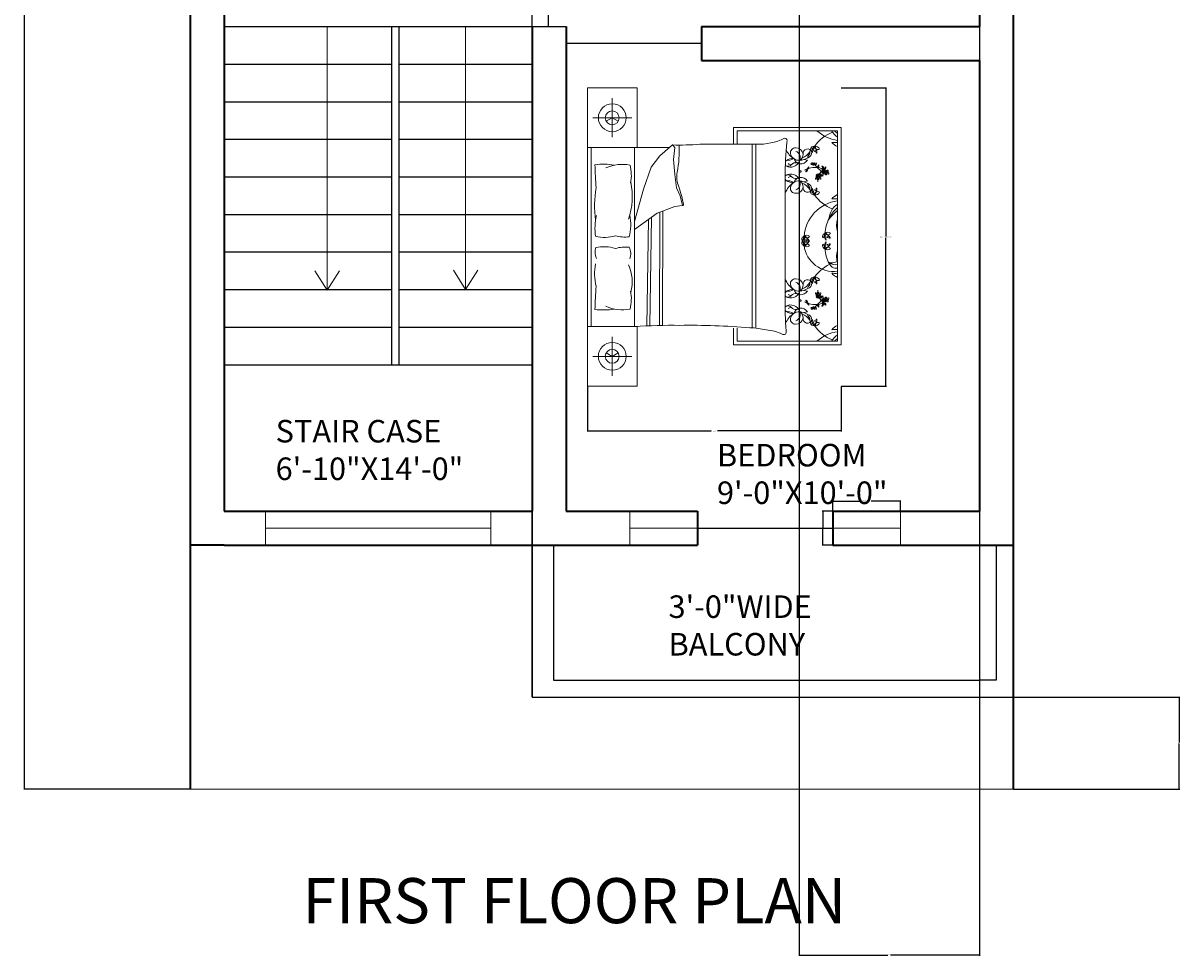
# Model space of a CAD drawing. Units: inches. Extents: x -16 to 587, y -783 to 64.
# Tile 8 of 14: x 279 to 587, y -782 to -534. Entities that reach past the tile are written whole.
import ezdxf

# ---------------------------------------------------------------- set-up
doc = ezdxf.new("R2010")
doc.units = ezdxf.units.IN
doc.header["$MEASUREMENT"] = 0
for name, color, linetype, lineweight in [('A-ANNO-DIMS', 2, 'Continuous', 18), ('A-ANNO-SYMB', 7, 'Continuous', 18), ('A-ANNO-TEXT', 7, 'Continuous', 25), ('A-AREA-IDEN', 7, 'Continuous', 18), ('A-DOOR', 3, 'Continuous', 25), ('A-FLOR-BALC', 7, 'Continuous', 25), ('A-FLOR-STRS', 7, 'Continuous', 25), ('A-FURN', 8, 'Continuous', 18), ('A-GLAZ', 4, 'Continuous', 18), ('A-WALL', 7, 'Continuous', 35), ('C-PROP', 7, 'Continuous', 18)]:
    doc.layers.add(name, color=color, linetype=linetype, lineweight=lineweight)
doc.styles.get("Standard").update_dxf_attribs({"font": 'arial.ttf'})
doc.dimstyles.get("Standard").update_dxf_attribs({"dimtxt": 0.18, "dimasz": 0.18, "dimexe": 0.18, "dimexo": 0.0625, "dimgap": 0.09, "dimtad": 0, "dimtih": 1, "dimtoh": 1, "dimdec": 0, "dimzin": 0, "dimdsep": 46, "dimlunit": 3, "dimtxsty": 'Standard', "dimcen": 0.09, "dimadec": 0, "dimazin": 0, "dimtfac": 1, "dimtdec": 0, "dimtofl": 0, "dimtmove": 0, "dimatfit": 3, "dimfxl": 1, "dimtolj": 1, "dimtzin": 0, "dimarcsym": 0})

# ---------------------------------------------------------------- blocks, each defined once
blk = doc.blocks.new('BED-DOUBLE-COMPACT')
for p, q in [((0, 79.37), (0, 0)), ((6.61, 66.25), (6.61, 76.62)), ((11.8, 71.43), (1.43, 71.43)), ((38.91, 68.89), (38.91, 64.4)), ((67.5, 68.89), (38.91, 68.89)), ((39.83, 64.41), (39.83, 67.97)), ((39.83, 67.97), (66.58, 67.97)), ((66.58, 67.97), (66.58, 11.95)), ((67.5, 11.03), (67.5, 68.89)), ((0, 63.5), (21.78, 63.5)), ((1.02, 15.87), (1.02, 63.5)), ((12.54, 63.5), (12.54, 15.87)), ((22.61, 64.21), (19.24, 61.31)), ((23.26, 63.56), (22.61, 64.21)), ((22.93, 60.35), (23.26, 63.56)), ((43.86, 15.51), (43.86, 64.41)), ((44.85, 15.44), (44.85, 64.41)), ((19.24, 61.31), (16.99, 58.26)), ((23.26, 56.33), (22.93, 60.35)), ((58.53, 60.15), (57.63, 60.33)), ((16.99, 58.26), (14.9, 52.47)), ((23.74, 52.79), (23.26, 56.33)), ((52.64, 23.57), (52.64, 55.8)), ((14.9, 52.47), (12.54, 43.82)), ((24.7, 50.7), (23.74, 52.79)), ((58.53, 54.61), (57.63, 54.43)), ((25.34, 48.13), (24.7, 50.7)), ((18.6, 46.04), (23.26, 47.81)), ((19.15, 16.16), (19.27, 46.3)), ((19.97, 16.15), (20.09, 46.61)), ((23.26, 47.81), (25.34, 48.13)), ((12.54, 41.69), (18.6, 46.04)), ((15.84, 16.09), (16.24, 44.34)), ((16.65, 16.12), (17.06, 44.94)), ((58.53, 25.32), (57.63, 25.49)), ((58.53, 19.77), (57.63, 19.6)), ((38.91, 15.43), (38.91, 11.03)), ((39.83, 11.95), (39.83, 15.45)), ((6.61, 13.12), (6.61, 2.75)), ((38.91, 11.03), (67.5, 11.03)), ((66.58, 11.95), (39.83, 11.95)), ((11.8, 7.94), (1.43, 7.94))]:
    blk.add_line(p, q)
for points in [[(13.23, 63.5), (13.23, 79.37), (0, 79.37)], [(6.61, 71.43), (5.01, 70.51)], [(6.61, 71.43), (8.22, 70.51)], [(0, 15.87), (13.23, 15.87), (13.23, 0), (0, 0)], [(6.61, 7.94), (5.01, 8.86)], [(6.61, 7.94), (8.22, 8.86)]]:
    blk.add_lwpolyline(points)
for points in [[(29.88, 64.37, -0.001242), (44.94, 64.41, 0.127202), (52.44, 66)], [(1.98, 58.94, -0.074897), (7.16, 58.84, 0.472817)], [(7.45, 40.06, -0.14099), (2.16, 39.9, -0.235245)], [(7.45, 36.67, 0.14099), (2.16, 36.83, 0.235245)], [(1.98, 20.43, 0.074897), (7.16, 20.53, -0.472817)], [(43.23, 15.54, -0.056112), (47.6, 14.96, -0.095341), (51.8, 13.84)]]:
    blk.add_lwpolyline(points, format="xyb")
for centre, radius in [((6.61, 71.43), 3.7), ((6.61, 71.43), 1.85), ((61.41, 55.57), 0.202), ((63.54, 56.89), 0.202), ((61.41, 24.36), 0.202), ((63.54, 23.03), 0.202), ((6.61, 7.94), 3.7), ((6.61, 7.94), 1.85)]:
    blk.add_circle(centre, radius)
for centre, radius, start, end in [((67.97, 75.69), 10.36, 228.1144, 262.255), ((69.36, 70.49), 5.05, 209.8884, 236.5383), ((70.3, 72.31), 6.29, 223.5186, 233.6964), ((52.39, 65.27), 0.732, 332.6588, 86.02), ((135.26, 56.74), 82.62, 174.3113, 180.6567), ((69, 57.96), 10.36, 111.4092, 145.6135), ((68.19, 67.66), 4.21, 221.0454, 247.4453), ((65.93, 79.2), 14.34, 266.3481, 272.5919), ((24.59, 136.98), 72.8, 268.447, 274.1706), ((-5.49, 62.85), 29.95, 348.6608, 2.5481), ((58.23, 65.58), 6.01, 206.7003, 236.3329), ((55.35, 62.08), 1.34, 88.9462, 185.5144), ((56.34, 62.49), 2.39, 193.079, 274.7067), ((55.54, 61.53), 1.9, 7.1143, 95.0551), ((54.82, 60.79), 1.84, 338.5779, 68.4181), ((55.12, 61.86), 2.31, 305.9599, 357.6409), ((55.97, 64.33), 3.75, 288.2955, 328.7386), ((58.6, 61.97), 1.19, 19.1312, 189.736), ((58.24, 62.25), 1.49, 285.6955, 4.031), ((60.21, 60.65), 1.58, 128.4175, 173.8338), ((59.89, 62.21), 0.73, 126.7319, 206.0245), ((60.24, 62.98), 0.859, 76.272, 177.0484), ((58.93, 64.73), 1.77, 284.7031, 328.6173), ((61.4, 62.48), 1.64, 125.7657, 194.5347), ((53.37, 65.38), 7.25, 332.8176, 347.4827), ((60.69, 62.69), 1.15, 20.9613, 102.2885), ((61.31, 63.84), 0.866, 181.7131, 301.5367), ((58.47, 62.09), 2.62, 2.0648, 41.1598), ((60.05, 63.06), 0.848, 316.2238, 62.3173), ((60.58, 62.55), 0.112, 20.2817, 316.2238), ((60.96, 62.18), 0.129, 168.5166, 2.0648), ((60.9, 62.19), 0.0625, 52.0591, 168.5166), ((-753.35, 15.19), 756.59, 2.85022, 3.31479), ((9.24, 48.82), 10.23, 78.2417, 114.8684), ((1.05, 56.11), 10.64, 348.9631, 14.8961), ((53.52, 59.3), 0.956, 206.442, 225.5483), ((53.52, 59.3), 0.956, 127.675, 149.9707), ((53.23, 63.38), 3.29, 260.8446, 301.1782), ((54.08, 60.83), 2.53, 240.8249, 340.7178), ((53.33, 59.71), 1.19, 246.1646, 318.4347), ((54.66, 57.53), 3.06, 85.2696, 124.215), ((54.54, 61.21), 2.28, 240.0851, 262.564), ((55.44, 57.84), 1.63, 74.8529, 138.4347), ((56.82, 61.14), 1.97, 196.8663, 330.0915), ((55.99, 59.89), 0.493, 254.8529, 12.6959), ((54.66, 57.53), 3.06, 53.6555, 57.2989), ((56.28, 64.36), 4.26, 273.4924, 303.7117), ((59.65, 59.15), 0.156, 125.0752, 284.7644), ((59.89, 59.21), 0.337, 127.3642, 168.4363), ((59.63, 59.48), 0.486, 277.4968, 341.2737), ((60.01, 59.25), 0.193, 88.1325, 178.8919), ((60.4, 59.04), 0.418, 136.3462, 189.6513), ((60.16, 59), 0.174, 189.6513, 312.3208), ((60.21, 59.49), 0.202, 183.2768, 356.7232), ((60.84, 59.12), 0.662, 164.2829, 186.9148), ((60.06, 59.12), 0.331, 312.3208, 40.2111), ((60.76, 59.49), 0.47, 201.6382, 274.947), ((60.14, 58.85), 0.614, 42.3896, 66.5724), ((66.33, 63.71), 7.54, 217.9541, 226.8459), ((60.58, 59.21), 0.334, 10.9597, 52.2379), ((60.79, 59.18), 0.155, 274.947, 37.5263), ((60.36, 59.37), 1.28, 313.6929, 321.7899), ((61.77, 58.5), 0.417, 115.5379, 168.6744), ((60.36, 59.1), 1.25, 329.344, 349.7412), ((59.36, 58.81), 2.24, 352.8698, 1.6736), ((62.5, 58.36), 0.226, 33.0979, 123.1364), ((57.53, 55.18), 5.91, 31.1156, 34.8118), ((62.18, 57.97), 0.611, 2.3172, 70.5201), ((30.21, 55.69), 6.46, 168.6608, 203.7384), ((53.52, 55.45), 0.956, 134.4517, 156.771), ((54.08, 53.93), 2.53, 19.2822, 119.1751), ((53.33, 55.05), 1.19, 41.5653, 113.8354), ((54.54, 53.55), 2.28, 97.436, 119.9149), ((55.44, 56.92), 1.63, 221.5653, 285.1471), ((56.82, 53.62), 1.97, 29.9085, 163.1337), ((56.64, 57.17), 0.249, 169.5864, 349.5616), ((56.74, 57.15), 0.153, 349.5616, 167.2949), ((60.73, 51.65), 6.57, 110.1059, 116.9968), ((58.53, 57.07), 0.417, 129.5056, 182.6421), ((57.33, 58.03), 1.25, 308.4388, 328.836), ((57.11, 59.05), 2.24, 296.5064, 305.3102), ((57.1, 57.9), 1.28, 336.3901, 344.4871), ((58.48, 57.57), 0.162, 83.9457, 185.6216), ((57.84, 57.73), 0.665, 328.836, 0.8141), ((58.18, 57.53), 0.381, 306.5232, 32.4668), ((58.64, 57.83), 0.162, 112.5583, 214.2343), ((58.53, 58.12), 0.381, 265.7131, 351.6568), ((58.2, 58.33), 0.665, 297.3659, 329.344), ((57.69, 58.9), 1.28, 313.6929, 321.7899), ((59.1, 58.03), 0.417, 115.5379, 168.6744), ((57.69, 58.63), 1.25, 329.344, 349.7412), ((60.73, 51.65), 6.57, 86.1723, 106.4158), ((56.69, 58.34), 2.24, 352.8698, 1.6736), ((61.09, 55.29), 0.337, 93.635, 168.4363), ((61.11, 57.11), 0.921, 253.6301, 325.4631), ((61.37, 55.83), 0.652, 82.0748, 142.6895), ((61.29, 56.73), 0.669, 228.342, 274.9894), ((61.05, 55.82), 0.198, 138.2946, 276.2474), ((61.13, 55.79), 0.276, 358.5719, 143.8954), ((61.22, 55.33), 0.193, 88.1325, 178.8919), ((61.29, 56.01), 0.278, 208.8493, 269.9355), ((61.05, 55.94), 0.318, 274.2123, 318.1587), ((61.31, 58.3), 0.162, 112.5583, 214.2343), ((61.2, 58.59), 0.381, 265.7131, 351.6568), ((60.87, 58.8), 0.665, 297.3659, 329.344), ((60.9, 54.92), 3.3, 60.7959, 85.244), ((53.88, 50.18), 10.84, 37.8256, 47.7588), ((61.31, 56.62), 0.56, 273.8774, 357.1501), ((62.02, 55.62), 0.637, 121.9501, 165.2442), ((61.53, 57.02), 0.542, 262.0748, 308.2393), ((61.58, 55.87), 0.134, 262.868, 7.094), ((61.34, 54.93), 0.614, 42.3896, 66.5724), ((61.56, 55.98), 0.399, 278.5614, 22.5914), ((61.78, 55.29), 0.334, 10.9597, 118.7804), ((65.28, 54.59), 3.95, 156.1523, 156.9499), ((61.79, 55.99), 0.2, 44.3732, 121.9501), ((62.4, 56.46), 0.56, 181.4625, 249.4747), ((65.28, 54.59), 3.95, 130.182, 149.456), ((62.31, 56.9), 0.542, 215.1128, 261.2773), ((62.74, 56.87), 0.921, 197.889, 269.722), ((62.46, 56.56), 0.669, 248.3627, 295.0101), ((62.13, 55.72), 0.652, 20.6625, 81.2773), ((63.1, 56.84), 0.652, 139.3812, 199.9959), ((61.88, 57.31), 0.921, 310.9365, 22.7695), ((62.31, 57.26), 0.669, 285.6484, 332.2957), ((62.68, 57.82), 0.176, 135.7354, 318.1297), ((62.39, 58.11), 0.234, 315.7354, 31.1156), ((62.19, 57.61), 0.542, 319.3812, 5.5456), ((62.81, 57.82), 0.176, 68.2452, 250.6395), ((62.41, 58.04), 0.526, 352.6008, 57.1845), ((64.29, 54.51), 3.52, 111.7087, 116.2181), ((60.9, 54.92), 3.3, 47.5083, 55.9967), ((62.91, 58.16), 0.526, 252.8042, 349.6943), ((62.41, 57.22), 0.56, 331.1838, 51.6792), ((62.98, 56.55), 0.156, 125.0752, 284.7644), ((62.97, 58.2), 0.234, 248.2452, 323.6254), ((63.22, 56.61), 0.337, 93.635, 168.4363), ((63.18, 57.14), 0.198, 138.2946, 276.2474), ((62.76, 58.35), 0.611, 291.7087, 3.0299), ((62.96, 56.88), 0.486, 277.4968, 341.2737), ((63.26, 57.11), 0.276, 358.5719, 143.8954), ((58.4, 61.57), 5.91, 323.6254, 327.3216), ((63.35, 56.65), 0.193, 88.1325, 178.8919), ((63.42, 57.33), 0.278, 208.8493, 269.9355), ((63.18, 57.26), 0.318, 274.2123, 318.1587), ((63.73, 56.45), 0.418, 136.3462, 189.6513), ((63.49, 56.41), 0.174, 189.6513, 312.3208), ((63.24, 58.19), 0.226, 325.6077, 55.6462), ((64.17, 56.53), 0.662, 164.2829, 186.9148), ((64.15, 56.94), 0.637, 121.9501, 165.2442), ((63.39, 56.52), 0.331, 312.3208, 40.2111), ((64.09, 56.9), 0.47, 201.6382, 274.947), ((63.71, 57.19), 0.134, 262.868, 7.094), ((63.47, 56.25), 0.614, 42.3896, 66.5724), ((63.69, 57.3), 0.399, 278.5614, 22.5914), ((63.91, 56.61), 0.334, 10.9597, 118.7804), ((63.92, 57.31), 0.2, 44.3732, 121.9501), ((64.12, 56.58), 0.155, 274.947, 37.5263), ((30.7, 48.06), 28.79, 170.503, 187.7804), ((-6.51, 50.51), 18.45, 340.7385, 11.9603), ((-4.65, 42.62), 30.78, 10.6617, 19.8806), ((53.52, 55.45), 0.956, 203.2856, 232.325), ((53.23, 51.38), 3.29, 58.8218, 100.2867), ((58.23, 49.18), 6.01, 123.6671, 158.5059), ((54.66, 57.23), 3.06, 235.785, 274.7304), ((56.34, 52.27), 2.39, 85.2933, 166.921), ((55.35, 52.68), 1.34, 174.4856, 271.0538), ((55.54, 53.23), 1.9, 264.9449, 352.8857), ((54.82, 53.97), 1.84, 291.5819, 21.4221), ((55.99, 54.87), 0.493, 347.3041, 105.1471), ((54.66, 57.23), 3.06, 302.7011, 306.3445), ((55.12, 52.9), 2.31, 2.3591, 54.0401), ((56.28, 50.39), 4.26, 56.2883, 86.5076), ((55.97, 50.43), 3.75, 31.2614, 71.7045), ((58.6, 52.79), 1.19, 170.264, 340.8688), ((60.21, 54.11), 1.58, 186.1662, 231.5825), ((58.24, 52.5), 1.49, 355.969, 74.3045), ((59.89, 52.54), 0.73, 153.9755, 233.2681), ((61.4, 52.28), 1.64, 165.4653, 234.2343), ((53.37, 49.37), 7.25, 12.5173, 27.1824), ((58.47, 52.67), 2.62, 318.8402, 357.9352), ((60.85, 55.23), 0.156, 125.0752, 284.7644), ((60.96, 52.58), 0.129, 357.9352, 191.4834), ((60.9, 52.57), 0.0625, 191.4834, 307.9409), ((60.83, 55.56), 0.486, 277.4968, 341.2737), ((61.6, 55.13), 0.418, 136.3462, 189.6513), ((61.36, 55.09), 0.174, 189.6513, 312.3208), ((65.28, 54.59), 3.95, 175.2415, 182.8929), ((62.04, 55.21), 0.662, 164.2829, 186.9148), ((61.26, 55.2), 0.331, 312.3208, 40.2111), ((61.96, 55.57), 0.47, 201.6382, 274.947), ((61.99, 55.26), 0.155, 274.947, 37.5263), ((67.97, 39.07), 10.36, 97.745, 175.5377), ((60.24, 51.78), 0.859, 182.9516, 283.728), ((58.93, 50.02), 1.77, 31.3827, 75.2969), ((60.05, 51.7), 0.848, 297.6827, 43.7762), ((61.31, 50.92), 0.866, 58.4633, 178.2869), ((60.69, 52.07), 1.15, 257.7115, 339.0387), ((69, 56.8), 10.36, 214.3865, 248.5908), ((60.54, 52.19), 0.0676, 43.7729, 339.7333), ((68.19, 47.1), 4.21, 112.5547, 138.9546), ((65.93, 35.55), 14.34, 87.4081, 93.6519), ((25.41, 48.31), 0.192, 250.2464, 1.1377), ((69.36, 44.27), 5.05, 123.4617, 178.728), ((70.3, 42.45), 6.29, 126.3036, 162.1496), ((72.07, 39.14), 9.36, 125.947, 145.9877), ((16.15, 41.98), 14.14, 166.04, 188.4751), ((-2.48, 43.04), 14, 346.3762, 10.1383), ((73.53, 39.86), 10.36, 152.5854, 175.5377), ((72.03, 42.76), 5.7, 162.9798, 196.4569), ((10.1, 49.41), 9.72, 254.1707, 275.9871), ((58.41, 39.02), 1.15, 50.8855, 132.2127), ((63.43, 39.84), 0.859, 106.1963, 206.9726), ((61.42, 40.71), 1.77, 314.6273, 358.5415), ((64.69, 39.99), 1.64, 155.6899, 224.4589), ((63.97, 39.82), 1.15, 50.8855, 132.2127), ((63.93, 41.12), 0.866, 211.6373, 331.4609), ((62.34, 38.19), 2.62, 31.989, 71.0841), ((56.27, 38.5), 7.25, 2.7418, 17.407), ((63.23, 39.82), 0.848, 346.148, 92.2415), ((74.96, 40.5), 8.43, 174.3643, 175.6213), ((80.74, 36.06), 15.06, 160.0972, 160.2783), ((10.1, 27.31), 9.72, 84.0129, 105.8293), ((7.31, 35.21), 4.21, 341.4593, 24.9817), ((57.88, 39.05), 0.859, 106.1963, 206.9726), ((57.88, 38.23), 0.859, 153.0274, 253.8037), ((55.87, 39.92), 1.77, 314.6273, 358.5415), ((55.87, 37.36), 1.77, 1.4585, 45.3727), ((59.14, 39.2), 1.64, 155.6899, 224.4589), ((59.14, 38.08), 1.64, 135.5411, 204.3101), ((58.38, 40.33), 0.866, 211.6373, 331.4609), ((50.72, 37.7), 7.25, 2.7418, 17.407), ((57.67, 39.03), 0.848, 346.148, 92.2415), ((56.79, 37.39), 2.62, 31.989, 71.0841), ((50.72, 39.57), 7.25, 342.593, 357.2582), ((56.79, 39.88), 2.62, 288.9159, 328.011), ((57.67, 38.25), 0.848, 267.7585, 13.852), ((58.38, 36.95), 0.866, 28.5391, 148.3627), ((58.41, 38.25), 1.15, 227.7873, 309.1145), ((65.58, 38.54), 8.02, 188.1803, 277.1364), ((58.39, 38.85), 0.112, 50.0755, 346.148), ((58.35, 38.44), 0.0676, 13.9791, 309.8091), ((58.91, 38.71), 0.129, 198.4408, 31.989), ((58.84, 38.69), 0.0625, 81.9833, 198.4408), ((58.91, 38.56), 0.129, 328.011, 161.5592), ((58.84, 38.58), 0.0625, 161.5592, 278.0167), ((63.43, 37.44), 0.859, 153.0274, 253.8037), ((61.42, 36.56), 1.77, 1.4585, 45.3727), ((64.69, 37.28), 1.64, 135.5411, 204.3101), ((56.27, 38.78), 7.25, 342.593, 357.2582), ((62.34, 39.09), 2.62, 288.9159, 328.011), ((63.23, 37.46), 0.848, 267.7585, 13.852), ((63.93, 36.16), 0.866, 28.5391, 148.3627), ((63.94, 39.64), 0.112, 50.0755, 346.148), ((63.9, 37.64), 0.0676, 13.9791, 309.8091), ((64.39, 39.49), 0.0625, 81.9833, 198.4408), ((64.39, 37.79), 0.0625, 161.5592, 278.0167), ((64.46, 39.51), 0.129, 198.4408, 31.989), ((64.46, 37.77), 0.129, 328.011, 161.5592), ((5.94, 35.74), 3.93, 163.8974, 206.6563), ((63.97, 37.46), 1.15, 227.7873, 309.1145), ((73.53, 37.42), 10.36, 184.4623, 207.4146), ((72.03, 34.52), 5.7, 163.5431, 197.0202), ((74.96, 36.78), 8.43, 184.3787, 185.6357), ((80.74, 41.21), 15.06, 199.7217, 199.9028), ((15.87, 29.85), 13.95, 168.8159, 193.6573), ((1.83, 27.85), 10.1, 343.8254, 26.1239), ((69, 23.12), 10.36, 111.4092, 145.6135), ((64.85, 37.51), 4.64, 263.3805, 291.883), ((66.14, 33.25), 1.86, 190.9261, 283.6102), ((65.88, 34.65), 2.35, 228.0951, 287.1391), ((58.23, 30.75), 6.01, 201.4941, 236.3329), ((55.35, 27.25), 1.34, 88.9462, 185.5144), ((55.54, 26.7), 1.9, 7.1143, 95.0551), ((58.6, 27.13), 1.19, 19.1312, 189.736), ((59.89, 27.38), 0.73, 126.7319, 206.0245), ((60.24, 28.14), 0.859, 76.272, 177.0484), ((58.93, 29.9), 1.77, 284.7031, 328.6173), ((61.4, 27.65), 1.64, 125.7657, 194.5347), ((53.37, 30.55), 7.25, 332.8176, 347.4827), ((60.69, 27.85), 1.15, 20.9613, 102.2885), ((60.05, 28.23), 0.848, 316.2238, 62.3173), ((58.47, 27.25), 2.62, 2.0648, 41.1598), ((61.31, 29), 0.866, 181.7131, 301.5367), ((60.58, 27.72), 0.112, 20.2817, 316.2238), ((65.93, 44.37), 14.34, 266.3481, 272.5919), ((68.19, 32.83), 4.21, 221.0454, 247.4453), ((-753.35, 64.18), 756.59, 356.68521, 357.14978), ((1.05, 23.26), 10.64, 345.1039, 11.0369), ((53.23, 28.54), 3.29, 259.7133, 301.1782), ((53.52, 24.47), 0.956, 127.675, 156.7144), ((54.08, 26), 2.53, 240.8249, 340.7178), ((54.66, 22.7), 3.06, 85.2696, 124.215), ((56.34, 27.66), 2.39, 193.079, 274.7067), ((56.82, 26.3), 1.97, 196.8663, 330.0915), ((54.82, 25.95), 1.84, 338.5779, 68.4181), ((55.99, 25.05), 0.493, 254.8529, 12.6959), ((54.66, 22.7), 3.06, 53.6555, 57.2989), ((55.12, 27.03), 2.31, 305.9599, 357.6409), ((56.28, 29.53), 4.26, 273.4924, 303.7117), ((55.97, 29.5), 3.75, 288.2955, 328.7386), ((58.24, 27.42), 1.49, 285.6955, 4.031), ((60.21, 25.82), 1.58, 128.4175, 173.8338), ((60.85, 24.7), 0.156, 75.2356, 234.9248), ((60.96, 27.34), 0.129, 168.5166, 2.0648), ((60.9, 27.35), 0.0625, 52.0591, 168.5166), ((60.83, 24.37), 0.486, 18.7263, 82.5032), ((61.36, 24.84), 0.174, 47.6792, 170.3487), ((61.6, 24.8), 0.418, 170.3487, 223.6538), ((65.28, 25.34), 3.95, 177.1071, 184.7585), ((62.04, 24.72), 0.662, 173.0852, 195.7171), ((61.26, 24.72), 0.331, 319.7889, 47.6792), ((61.96, 24.35), 0.47, 85.053, 158.3618), ((61.99, 24.66), 0.155, 322.4737, 85.053), ((129.84, 21.14), 77.23, 178.1965, 184.7598), ((53.52, 24.47), 0.956, 203.2856, 225.5483), ((53.33, 24.87), 1.19, 246.1646, 318.4347), ((54.08, 19.09), 2.53, 19.2822, 119.1751), ((54.54, 26.38), 2.28, 240.0851, 262.564), ((55.44, 23.01), 1.63, 74.8529, 138.4347), ((56.64, 22.76), 0.249, 10.4384, 190.4136), ((56.74, 22.77), 0.153, 192.7051, 10.4384), ((60.73, 28.27), 6.57, 243.0032, 249.8941), ((57.33, 21.89), 1.25, 31.164, 51.5612), ((58.53, 22.86), 0.417, 177.3579, 230.4944), ((57.11, 20.87), 2.24, 54.6898, 63.4936), ((57.1, 22.02), 1.28, 15.5129, 23.6099), ((58.48, 22.35), 0.162, 174.3784, 276.0543), ((58.18, 22.39), 0.381, 327.5332, 53.4768), ((57.84, 22.2), 0.665, 359.1859, 31.164), ((58.64, 22.1), 0.162, 145.7657, 247.4417), ((58.53, 21.81), 0.381, 8.3432, 94.2869), ((58.2, 21.6), 0.665, 30.656, 62.6341), ((57.69, 21.03), 1.28, 38.2101, 46.3071), ((59.1, 21.9), 0.417, 191.3256, 244.4621), ((57.69, 21.3), 1.25, 10.2588, 30.656), ((60.73, 28.27), 6.57, 253.5842, 273.8277), ((56.69, 21.59), 2.24, 358.3264, 7.1302), ((66.33, 16.22), 7.54, 133.1541, 142.0459), ((61.09, 24.64), 0.337, 191.5637, 266.365), ((61.05, 24.1), 0.198, 83.7526, 221.7054), ((61.29, 23.19), 0.669, 85.0106, 131.658), ((61.11, 22.81), 0.921, 34.5369, 106.3699), ((61.37, 24.09), 0.652, 217.3105, 277.9252), ((61.13, 24.13), 0.276, 216.1046, 1.4281), ((61.22, 24.59), 0.193, 181.1081, 271.8675), ((61.29, 23.92), 0.278, 90.0645, 151.1507), ((61.05, 23.98), 0.318, 41.8413, 85.7877), ((61.31, 21.62), 0.162, 145.7657, 247.4417), ((53.88, 29.74), 10.84, 312.2412, 322.1744), ((60.9, 25), 3.3, 274.756, 299.2041), ((61.2, 21.33), 0.381, 8.3432, 94.2869), ((60.87, 21.12), 0.665, 30.656, 62.6341), ((61.31, 23.3), 0.56, 2.8499, 86.1226), ((62.02, 24.3), 0.637, 194.7558, 238.0499), ((61.53, 22.91), 0.542, 51.7607, 97.9252), ((61.58, 24.06), 0.134, 352.906, 97.132), ((61.34, 24.99), 0.614, 293.4276, 317.6104), ((61.78, 24.63), 0.334, 241.2196, 349.0403), ((61.56, 23.94), 0.399, 337.4086, 81.4386), ((65.28, 25.34), 3.95, 203.0501, 203.8477), ((61.79, 23.93), 0.2, 238.0499, 315.6268), ((62.4, 23.46), 0.56, 110.5253, 178.5375), ((62.74, 23.05), 0.921, 90.278, 162.111), ((62.31, 23.02), 0.542, 98.7227, 144.8872), ((65.28, 25.34), 3.95, 210.544, 229.818), ((62.46, 23.36), 0.669, 64.9899, 111.6373), ((62.13, 24.2), 0.652, 278.7227, 339.3375), ((62.18, 21.95), 0.611, 289.4799, 357.6828), ((57.53, 24.75), 5.91, 325.1882, 328.8844), ((63.1, 23.09), 0.652, 160.0041, 220.6188), ((61.88, 22.61), 0.921, 337.2305, 49.0635), ((62.31, 22.66), 0.669, 27.7043, 74.3516), ((62.68, 22.1), 0.176, 41.8703, 224.2646), ((62.39, 21.82), 0.234, 328.8844, 44.2646), ((62.19, 22.31), 0.542, 354.4544, 40.6188), ((62.81, 22.1), 0.176, 109.3605, 291.7548), ((62.41, 21.88), 0.526, 302.8155, 7.3992), ((64.29, 25.42), 3.52, 243.7819, 248.2913), ((60.9, 25), 3.3, 304.0033, 312.4917), ((62.41, 22.71), 0.56, 308.3208, 28.8162), ((62.91, 21.76), 0.526, 10.3057, 107.1958), ((62.98, 23.37), 0.156, 75.2356, 234.9248), ((62.97, 21.72), 0.234, 36.3746, 111.7548), ((63.22, 23.31), 0.337, 191.5637, 266.365), ((63.18, 22.78), 0.198, 83.7526, 221.7054), ((62.76, 21.58), 0.611, 356.9701, 68.2913), ((62.96, 23.04), 0.486, 18.7263, 82.5032), ((63.26, 22.81), 0.276, 216.1046, 1.4281), ((63.35, 23.27), 0.193, 181.1081, 271.8675), ((58.4, 18.36), 5.91, 32.6784, 36.3746), ((63.42, 22.59), 0.278, 90.0645, 151.1507), ((63.18, 22.66), 0.318, 41.8413, 85.7877), ((63.49, 23.52), 0.174, 47.6792, 170.3487), ((63.73, 23.47), 0.418, 170.3487, 223.6538), ((63.24, 21.73), 0.226, 304.3538, 34.3923), ((64.17, 23.4), 0.662, 173.0852, 195.7171), ((64.15, 22.98), 0.637, 194.7558, 238.0499), ((63.39, 23.4), 0.331, 319.7889, 47.6792), ((64.09, 23.03), 0.47, 85.053, 158.3618), ((63.71, 22.74), 0.134, 352.906, 97.132), ((63.47, 23.67), 0.614, 293.4276, 317.6104), ((63.91, 23.31), 0.334, 241.2196, 349.0403), ((63.69, 22.62), 0.399, 337.4086, 81.4386), ((63.92, 22.61), 0.2, 238.0499, 315.6268), ((64.12, 23.34), 0.155, 322.4737, 85.053), ((9.24, 30.54), 10.23, 245.1316, 281.7583), ((53.52, 20.62), 0.956, 134.4517, 163.3657), ((53.52, 20.62), 0.956, 197.4186, 232.325), ((53.23, 16.55), 3.29, 58.8218, 100.751), ((58.23, 14.34), 6.01, 123.6671, 156.3547), ((53.33, 20.22), 1.19, 41.5653, 113.8354), ((54.66, 22.39), 3.06, 235.785, 274.7304), ((54.54, 18.71), 2.28, 97.436, 119.9149), ((56.34, 17.43), 2.39, 85.2933, 166.921), ((55.44, 22.08), 1.63, 221.5653, 285.1471), ((56.82, 18.79), 1.97, 29.9085, 163.1337), ((54.82, 19.14), 1.84, 291.5819, 21.4221), ((55.99, 20.04), 0.493, 347.3041, 105.1471), ((54.66, 22.39), 3.06, 302.7011, 306.3445), ((55.12, 18.06), 2.31, 2.3591, 54.0401), ((56.28, 15.56), 4.26, 56.2883, 86.5076), ((55.97, 15.59), 3.75, 31.2614, 71.7045), ((58.24, 17.67), 1.49, 355.969, 74.3045), ((60.21, 19.27), 1.58, 186.1662, 231.5825), ((59.65, 20.78), 0.156, 75.2356, 234.9248), ((59.89, 20.72), 0.337, 191.5637, 232.6358), ((59.63, 20.45), 0.486, 18.7263, 82.5032), ((60.01, 20.67), 0.193, 181.1081, 271.8675), ((60.16, 20.92), 0.174, 47.6792, 170.3487), ((60.4, 20.88), 0.418, 170.3487, 223.6538), ((60.21, 20.44), 0.202, 3.2768, 176.7232), ((60.84, 20.8), 0.662, 173.0852, 195.7171), ((60.06, 20.8), 0.331, 319.7889, 47.6792), ((60.76, 20.43), 0.47, 85.053, 158.3618), ((60.14, 21.07), 0.614, 293.4276, 317.6104), ((60.58, 20.71), 0.334, 307.7621, 349.0403), ((60.79, 20.74), 0.155, 322.4737, 85.053), ((60.36, 20.55), 1.28, 38.2101, 46.3071), ((61.77, 21.42), 0.417, 191.3256, 244.4621), ((60.36, 20.82), 1.25, 10.2588, 30.656), ((59.36, 21.11), 2.24, 358.3264, 7.1302), ((62.5, 21.56), 0.226, 236.8636, 326.9021), ((22.24, -126.41), 142.61, 89.0718, 93.9), ((27.43, -169.82), 186.03, 85.1265, 90.8855), ((55.35, 17.84), 1.34, 174.4856, 271.0538), ((55.54, 18.39), 1.9, 264.9449, 352.8857), ((58.6, 17.96), 1.19, 170.264, 340.8688), ((59.89, 17.71), 0.73, 153.9755, 233.2681), ((58.93, 15.19), 1.77, 31.3827, 75.2969), ((60.24, 16.95), 0.859, 182.9516, 283.728), ((61.4, 17.44), 1.64, 165.4653, 234.2343), ((53.37, 14.54), 7.25, 12.5173, 27.1824), ((58.47, 17.84), 2.62, 318.8402, 357.9352), ((60.05, 16.86), 0.848, 297.6827, 43.7762), ((61.31, 16.09), 0.866, 58.4633, 178.2869), ((60.69, 17.24), 1.15, 257.7115, 339.0387), ((69, 21.97), 10.36, 214.3865, 248.5908), ((60.54, 17.36), 0.0676, 43.7729, 339.7333), ((60.96, 17.75), 0.129, 357.9352, 191.4834), ((60.9, 17.73), 0.0625, 191.4834, 307.9409), ((68.19, 12.26), 4.21, 112.5547, 138.9546), ((52.21, 14.44), 0.723, 236.1736, 23.4781), ((67.97, 4.23), 10.36, 97.745, 131.8856), ((69.36, 9.43), 5.05, 123.4617, 150.1116), ((65.93, 0.72), 14.34, 87.4081, 93.6519), ((70.3, 7.62), 6.29, 126.3036, 136.4814)]:
    blk.add_arc(centre, radius, start, end)
blk = doc.blocks.new('WIN-60')
for p, q in [((0, 9), (60, 9)), ((0, 0), (0, 9)), ((60, 9), (60, 0)), ((0, 4.5), (60, 4.5)), ((60, 0), (0, 0))]:
    blk.add_line(p, q)
blk = doc.blocks.new('WIN-18')
for p, q in [((18, 9), (0, 9)), ((0, 9), (0, 0)), ((18, 0), (18, 9)), ((18, 4.5), (0, 4.5)), ((0, 0), (18, 0))]:
    blk.add_line(p, q)
blk = doc.blocks.new('STAIR-DIRECTION')
for p, q in [((3.25, 70), (3.25, 0)), ((3.25, 0), (0, 5.12)), ((3.25, 0), (6.51, 5.12))]:
    blk.add_line(p, q)
blk = doc.blocks.new('*D32')
at = {"layer": 'A-ANNO-DIMS', "color": 0, "lineweight": -2, "transparency": 16777216}
for p, q in [((497.03, -550.9), (509.05, -550.9)), ((508.87, -551.08), (508.87, -590.4)), ((508.87, -630.09), (508.87, -590.77)), ((497.03, -630.27), (509.05, -630.27))]:
    blk.add_line(p, q, dxfattribs=at)
at = {"layer": 'A-ANNO-DIMS', "color": 0, "transparency": 16777216}
for points in [[(508.84, -551.08), (508.9, -551.08), (508.87, -550.9)], [(508.84, -630.09), (508.9, -630.09), (508.87, -630.27)]]:
    blk.add_solid(points, dxfattribs=at)
at = {"layer": 'Defpoints', "color": 0, "transparency": 16777216}
for p in [(496.97, -550.9), (508.87, -550.9), (496.97, -630.27)]:
    blk.add_point(p, dxfattribs=at)
at = {"layer": 'A-ANNO-DIMS', "color": 0, "transparency": 16777216, "insert": (508.87, -590.59), "char_height": 0.18, "attachment_point": 5}
blk.add_mtext('\\A1;DOUBLE BED 6\'-7 1/2" TYP.', dxfattribs=at)
blk = doc.blocks.new('*D33')
at = {"layer": 'A-ANNO-DIMS', "color": 0, "lineweight": -2, "transparency": 16777216}
for p, q in [((429.47, -630.33), (429.47, -642.35)), ((496.97, -630.33), (496.97, -642.35)), ((429.65, -642.17), (462.37, -642.17)), ((496.79, -642.17), (464.07, -642.17))]:
    blk.add_line(p, q, dxfattribs=at)
at = {"layer": 'A-ANNO-DIMS', "color": 0, "transparency": 16777216}
for points in [[(429.65, -642.14), (429.65, -642.2), (429.47, -642.17)], [(496.79, -642.14), (496.79, -642.2), (496.97, -642.17)]]:
    blk.add_solid(points, dxfattribs=at)
at = {"layer": 'Defpoints', "color": 0, "transparency": 16777216}
for p in [(429.47, -630.27), (496.97, -630.27), (496.97, -642.17)]:
    blk.add_point(p, dxfattribs=at)
at = {"layer": 'A-ANNO-DIMS', "color": 0, "transparency": 16777216, "insert": (463.22, -642.17), "char_height": 0.18, "attachment_point": 5}
blk.add_mtext('\\A1;5\'-7 1/2" TYP.', dxfattribs=at)
blk = doc.blocks.new('*D50')
at = {"layer": 'A-ANNO-DIMS', "color": 0, "lineweight": -2, "transparency": 16777216}
for p, q in [((494.79, -663.49), (494.79, -660.67)), ((494.97, -660.85), (502.56, -660.85)), ((512.61, -660.85), (505.02, -660.85)), ((512.79, -663.49), (512.79, -660.67))]:
    blk.add_line(p, q, dxfattribs=at)
at = {"layer": 'A-ANNO-DIMS', "color": 0, "transparency": 16777216}
for points in [[(494.97, -660.82), (494.97, -660.88), (494.79, -660.85)], [(512.61, -660.82), (512.61, -660.88), (512.79, -660.85)]]:
    blk.add_solid(points, dxfattribs=at)
at = {"layer": 'Defpoints', "color": 0, "transparency": 16777216}
for p in [(512.79, -660.85), (494.79, -663.55), (512.79, -663.55)]:
    blk.add_point(p, dxfattribs=at)
at = {"layer": 'A-ANNO-DIMS', "color": 0, "transparency": 16777216, "insert": (503.79, -660.85), "char_height": 0.18, "attachment_point": 5}
blk.add_mtext('\\A1;WINDOW 1\'-6" TYP.', dxfattribs=at)
blk = doc.blocks.new('*D51')
at = {"layer": 'A-ANNO-DIMS', "color": 0, "lineweight": -2, "transparency": 16777216}
for p, q in [((494.73, -663.55), (491.91, -663.55)), ((492.09, -663.73), (492.09, -667.87)), ((492.09, -672.37), (492.09, -668.24)), ((494.73, -672.55), (491.91, -672.55))]:
    blk.add_line(p, q, dxfattribs=at)
at = {"layer": 'A-ANNO-DIMS', "color": 0, "transparency": 16777216}
for points in [[(492.06, -663.73), (492.12, -663.73), (492.09, -663.55)], [(492.06, -672.37), (492.12, -672.37), (492.09, -672.55)]]:
    blk.add_solid(points, dxfattribs=at)
at = {"layer": 'Defpoints', "color": 0, "transparency": 16777216}
for p in [(492.09, -663.55), (494.79, -663.55), (494.79, -672.55)]:
    blk.add_point(p, dxfattribs=at)
at = {"layer": 'A-ANNO-DIMS', "color": 0, "transparency": 16777216, "insert": (492.09, -668.05), "char_height": 0.18, "attachment_point": 5}
blk.add_mtext('\\A1;0\'-9" TYP.', dxfattribs=at)
blk = doc.blocks.new('*D53')
at = {"layer": 'A-ANNO-DIMS', "color": 0, "lineweight": -2, "transparency": 16777216}
for p, q in [((323.73, 19.45), (279.46, 19.45)), ((279.64, 19.27), (279.64, -358.87)), ((279.64, -737.37), (279.64, -359.24)), ((323.73, -737.55), (279.46, -737.55))]:
    blk.add_line(p, q, dxfattribs=at)
at = {"layer": 'A-ANNO-DIMS', "color": 0, "transparency": 16777216}
for points in [[(279.61, 19.27), (279.67, 19.27), (279.64, 19.45)], [(279.61, -737.37), (279.67, -737.37), (279.64, -737.55)]]:
    blk.add_solid(points, dxfattribs=at)
at = {"layer": 'Defpoints', "color": 0, "transparency": 16777216}
for p in [(323.79, 19.45), (279.64, -737.55), (323.79, -737.55)]:
    blk.add_point(p, dxfattribs=at)
at = {"layer": 'A-ANNO-DIMS', "color": 0, "transparency": 16777216, "insert": (279.64, -359.05), "char_height": 0.18, "attachment_point": 5}
blk.add_mtext('\\A1;63\'-1"', dxfattribs=at)
blk = doc.blocks.new('*D55')
at = {"layer": 'A-ANNO-DIMS', "color": 0, "lineweight": -2, "transparency": 16777216}
for p, q in [((485.79, -75.62), (485.79, -781.88)), ((533.79, -75.62), (533.79, -781.88)), ((485.97, -781.7), (509.46, -781.7)), ((533.61, -781.7), (510.12, -781.7))]:
    blk.add_line(p, q, dxfattribs=at)
at = {"layer": 'A-ANNO-DIMS', "color": 0, "transparency": 16777216}
for points in [[(485.97, -781.67), (485.97, -781.73), (485.79, -781.7)], [(533.61, -781.67), (533.61, -781.73), (533.79, -781.7)]]:
    blk.add_solid(points, dxfattribs=at)
at = {"layer": 'Defpoints', "color": 0, "transparency": 16777216}
for p in [(485.79, -75.55), (533.79, -75.55), (533.79, -781.7)]:
    blk.add_point(p, dxfattribs=at)
at = {"layer": 'A-ANNO-DIMS', "color": 0, "transparency": 16777216, "insert": (509.79, -781.7), "char_height": 0.18, "attachment_point": 5}
blk.add_mtext('\\A1;4\'-0"', dxfattribs=at)
blk = doc.blocks.new('*D59')
at = {"layer": 'A-ANNO-DIMS', "color": 0, "lineweight": -2, "transparency": 16777216}
for p, q in [((414.79, -712.99), (414.79, 63.78)), ((414.97, 63.6), (478.4, 63.6)), ((542.61, 63.6), (479.18, 63.6)), ((542.79, -712.99), (542.79, 63.78))]:
    blk.add_line(p, q, dxfattribs=at)
at = {"layer": 'A-ANNO-DIMS', "color": 0, "transparency": 16777216}
for points in [[(414.97, 63.63), (414.97, 63.57), (414.79, 63.6)], [(542.61, 63.63), (542.61, 63.57), (542.79, 63.6)]]:
    blk.add_solid(points, dxfattribs=at)
at = {"layer": 'Defpoints', "color": 0, "transparency": 16777216}
for p in [(542.79, 63.6), (414.79, -713.05), (542.79, -713.05)]:
    blk.add_point(p, dxfattribs=at)
at = {"layer": 'A-ANNO-DIMS', "color": 0, "transparency": 16777216, "insert": (478.79, 63.6), "char_height": 0.18, "attachment_point": 5}
blk.add_mtext('\\A1;10\'-8"', dxfattribs=at)
blk = doc.blocks.new('*D60')
at = {"layer": 'A-ANNO-DIMS', "color": 0, "lineweight": -2, "transparency": 16777216}
for p, q in [((542.85, -713.05), (587.12, -713.05)), ((586.94, -713.23), (586.94, -725.12)), ((586.94, -737.37), (586.94, -725.49)), ((542.85, -737.55), (587.12, -737.55))]:
    blk.add_line(p, q, dxfattribs=at)
at = {"layer": 'A-ANNO-DIMS', "color": 0, "transparency": 16777216}
for points in [[(586.91, -713.23), (586.97, -713.23), (586.94, -713.05)], [(586.91, -737.37), (586.97, -737.37), (586.94, -737.55)]]:
    blk.add_solid(points, dxfattribs=at)
at = {"layer": 'Defpoints', "color": 0, "transparency": 16777216}
for p in [(542.79, -713.05), (542.79, -737.55), (586.94, -737.55)]:
    blk.add_point(p, dxfattribs=at)
at = {"layer": 'A-ANNO-DIMS', "color": 0, "transparency": 16777216, "insert": (586.94, -725.3), "char_height": 0.18, "attachment_point": 5}
blk.add_mtext('\\A1;2\'-0 1/2"', dxfattribs=at)

msp = doc.modelspace()

# ---------------------------------------------------------------- linework, layer by layer
at = {"layer": 'A-DOOR'}
for p, q in [((419.12, -534.55), (419.12, -495.55)), ((459.79, -539.05), (423.79, -539.05)), ((458.79, -668.05), (494.79, -668.05))]:
    msp.add_line(p, q, dxfattribs=at)
at = {"layer": 'A-FLOR-BALC'}
for p, q in [((414.79, -663.55), (414.79, -713.05)), ((420.43, -672.55), (420.43, -708.55)), ((538.29, -672.55), (538.29, -708.55)), ((420.43, -708.55), (476.79, -708.55)), ((476.79, -708.55), (533.79, -708.55)), ((538.29, -708.55), (533.79, -708.55)), ((414.79, -713.05), (476.79, -713.05)), ((476.79, -713.05), (542.79, -713.05))]:
    msp.add_line(p, q, dxfattribs=at)
at = {"layer": 'A-FLOR-STRS'}
for p, q in [((332.79, -534.55), (423.79, -534.55)), ((377.29, -534.55), (377.29, -624.55)), ((379.29, -534.55), (379.29, -624.55)), ((332.79, -544.55), (377.29, -544.55)), ((379.29, -544.55), (414.79, -544.55)), ((332.79, -554.55), (377.29, -554.55)), ((379.29, -554.55), (414.79, -554.55)), ((332.79, -564.55), (377.29, -564.55)), ((379.29, -564.55), (414.79, -564.55)), ((332.79, -574.55), (377.29, -574.55)), ((379.29, -574.55), (414.79, -574.55)), ((332.79, -584.55), (377.29, -584.55)), ((379.29, -584.55), (414.79, -584.55)), ((332.79, -594.55), (377.29, -594.55)), ((379.29, -594.55), (414.79, -594.55)), ((332.79, -604.55), (377.29, -604.55)), ((379.29, -604.55), (414.79, -604.55)), ((332.79, -614.55), (377.29, -614.55)), ((379.29, -614.55), (414.79, -614.55)), ((332.79, -624.55), (414.79, -624.55))]:
    msp.add_line(p, q, dxfattribs=at)
at = {"layer": 'A-WALL'}
for p, q in [((323.79, 19.45), (323.79, -737.55)), ((542.79, 19.45), (542.79, -737.55)), ((332.79, -495.55), (332.79, -663.55)), ((533.79, -495.55), (533.79, -534.55)), ((414.79, -534.55), (414.79, -543.55)), ((423.79, -534.55), (423.79, -543.55)), ((459.79, -534.55), (459.79, -543.55)), ((459.79, -534.55), (476.79, -534.55)), ((476.79, -534.55), (533.79, -534.55)), ((414.79, -543.55), (414.79, -663.55)), ((423.79, -543.55), (423.79, -663.55)), ((459.79, -543.55), (476.79, -543.55)), ((476.79, -543.55), (533.79, -543.55)), ((533.79, -543.55), (533.79, -663.55)), ((332.79, -663.55), (414.79, -663.55)), ((423.79, -663.55), (458.79, -663.55)), ((458.79, -663.55), (458.79, -672.55)), ((494.79, -663.55), (533.79, -663.55)), ((494.79, -663.55), (494.79, -672.55)), ((332.79, -672.55), (323.79, -672.55)), ((332.79, -672.55), (458.79, -672.55)), ((494.79, -672.55), (533.79, -672.55)), ((533.79, -672.55), (542.79, -672.55))]:
    msp.add_line(p, q, dxfattribs=at)
at = {"layer": 'C-PROP'}
msp.add_line((323.79, -737.55), (542.79, -737.55), dxfattribs=at)

# ---------------------------------------------------------------- block references
at = {"layer": 'A-ANNO-SYMB'}
for p in [(356.94, -604.71), (393.79, -604.55)]:
    msp.add_blockref('STAIR-DIRECTION', p, dxfattribs=at)
at = {"layer": 'A-FURN'}
msp.add_blockref('BED-DOUBLE-COMPACT', (429.47, -630.27), dxfattribs=at)
at = {"layer": 'A-GLAZ', "rotation": 180}
msp.add_blockref('WIN-60', (403.79, -663.55), dxfattribs=at)
at = {"layer": 'A-GLAZ'}
for p in [(440.79, -672.55), (494.79, -672.55)]:
    msp.add_blockref('WIN-18', p, dxfattribs=at)

# ---------------------------------------------------------------- texts
at = {"layer": 'A-ANNO-TEXT', "insert": (353.59, -761.2), "char_height": 12, "attachment_point": 1}
msp.add_mtext('FIRST FLOOR PLAN', dxfattribs=at)
at = {"layer": 'A-AREA-IDEN', "char_height": 6, "attachment_point": 1}
for s, insert in [('STAIR CASE\\P6\'-10"X14\'-0"', (346.49, -639.25)), ('BEDROOM\\P9\'-0"X10\'-0"', (463.94, -645.63)), ('3\'-0"WIDE\\PBALCONY', (451.06, -685.95))]:
    msp.add_mtext(s, dxfattribs=dict(at, insert=insert))

# ---------------------------------------------------------------- dimensions: what is measured, and where the dimension line sits
at = {"layer": 'A-ANNO-DIMS'}
for base, p1, p2, picture, middle in [((542.79, 63.6), (414.79, -713.05), (542.79, -713.05), '*D59', (478.79, 63.6)), ((533.79, -781.7), (485.79, -75.55), (533.79, -75.55), '*D55', (509.79, -781.7))]:
    dim = msp.add_linear_dim(base=base, p1=p1, p2=p2, dimstyle='Standard', override={"dimdec": 1, "dimlfac": 1, "dimrnd": 0, "dimzin": 1, "dimdsep": 46, "dimlunit": 4, "dimfrac": 2}, dxfattribs=at)
    dim.commit()
    dim.dimension.update_dxf_attribs({"geometry": picture, "text_midpoint": middle})
for base, p1, p2, picture, middle in [((279.64, -737.55), (323.79, 19.45), (323.79, -737.55), '*D53', (279.64, -359.05)), ((586.94, -737.55), (542.79, -713.05), (542.79, -737.55), '*D60', (586.94, -725.3))]:
    dim = msp.add_linear_dim(base=base, p1=p1, p2=p2, angle=90, dimstyle='Standard', override={"dimdec": 1, "dimlfac": 1, "dimrnd": 0, "dimzin": 1, "dimdsep": 46, "dimlunit": 4, "dimfrac": 2}, dxfattribs=at)
    dim.commit()
    dim.dimension.update_dxf_attribs({"geometry": picture, "text_midpoint": middle})
for base, p1, p2, text, picture, middle in [((508.87, -550.9), (496.97, -630.27), (496.97, -550.9), 'DOUBLE BED <> TYP.', '*D32', (508.87, -590.59)), ((492.09, -663.55), (494.79, -672.55), (494.79, -663.55), '<> TYP.', '*D51', (492.09, -668.05))]:
    dim = msp.add_linear_dim(base=base, p1=p1, p2=p2, angle=90, text=text, dimstyle='Standard', override={"dimdec": 1, "dimlfac": 1, "dimrnd": 0, "dimzin": 1, "dimdsep": 46, "dimlunit": 4, "dimfrac": 2}, dxfattribs=at)
    dim.commit()
    dim.dimension.update_dxf_attribs({"geometry": picture, "text_midpoint": middle})
for base, p1, p2, text, picture, middle in [((496.97, -642.17), (429.47, -630.27), (496.97, -630.27), '<> TYP.', '*D33', (463.22, -642.17)), ((512.79, -660.85), (494.79, -663.55), (512.79, -663.55), 'WINDOW <> TYP.', '*D50', (503.79, -660.85))]:
    dim = msp.add_linear_dim(base=base, p1=p1, p2=p2, text=text, dimstyle='Standard', override={"dimdec": 1, "dimlfac": 1, "dimrnd": 0, "dimzin": 1, "dimdsep": 46, "dimlunit": 4, "dimfrac": 2}, dxfattribs=at)
    dim.commit()
    dim.dimension.update_dxf_attribs({"geometry": picture, "text_midpoint": middle})

doc.saveas('drawing.dxf')
